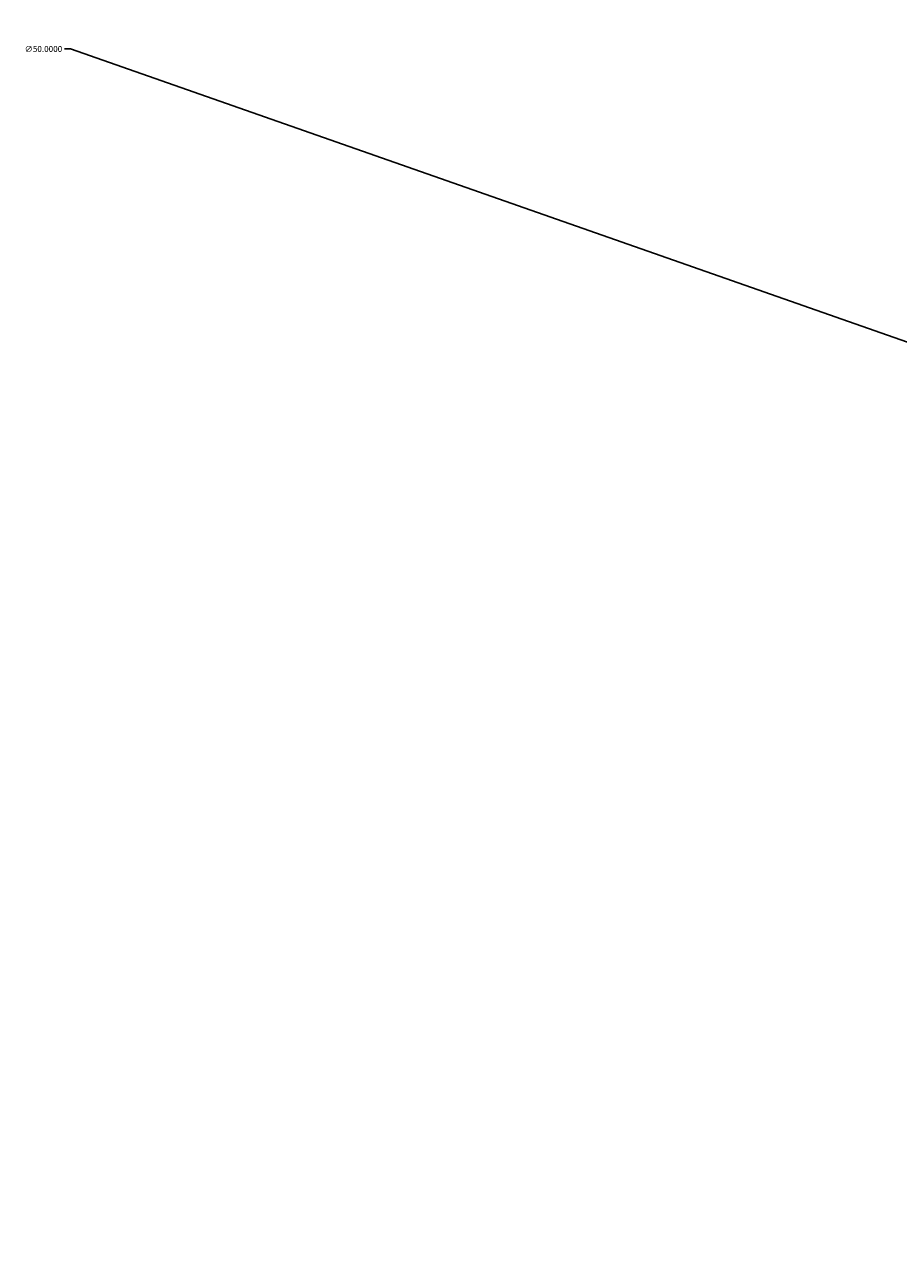
# Model space of a CAD drawing. Units: inches. Extents: x 139261 to 139415, y 52839 to 52963.
# Tile 3 of 20: x 139261 to 139288, y 52891 to 52928. Entities that reach past the tile are written whole.
import ezdxf

# ---------------------------------------------------------------- set-up
doc = ezdxf.new("R2010")
doc.units = ezdxf.units.IN
doc.header["$MEASUREMENT"] = 0
doc.layers.add('M-DIMS', color=2, linetype='Continuous', lineweight=25)
doc.styles.get("Standard").update_dxf_attribs({"font": 'arial.ttf'})
doc.dimstyles.get("Standard").update_dxf_attribs({"dimtxt": 0.18, "dimasz": 0.18, "dimexe": 0.18, "dimexo": 0.0625, "dimgap": 0.09, "dimtad": 0, "dimtih": 1, "dimtoh": 1, "dimdec": 4, "dimzin": 0, "dimdsep": 46, "dimtxsty": 'Standard', "dimcen": 0.09, "dimadec": 0, "dimazin": 0, "dimtfac": 1, "dimtdec": 4, "dimtofl": 0, "dimtmove": 0, "dimatfit": 3, "dimfxl": 1, "dimtolj": 1, "dimtzin": 0, "dimarcsym": 0})

# ---------------------------------------------------------------- blocks, each defined once
blk = doc.blocks.new('*D5')
at = {"layer": 'Defpoints', "color": 0, "transparency": 16777216}
for p in [(139316.763, 52908.484), (139363.951, 52891.951)]:
    blk.add_point(p, dxfattribs=at)
at = {"layer": 'M-DIMS', "color": 0, "lineweight": -2, "transparency": 16777216}
for p, q in [((139262.553, 52927.414), (139262.733, 52927.414)), ((139262.733, 52927.414), (139316.593, 52908.544)), ((139340.267, 52900.217), (139340.447, 52900.217)), ((139340.357, 52900.127), (139340.357, 52900.307))]:
    blk.add_line(p, q, dxfattribs=at)
at = {"layer": 'M-DIMS', "color": 0, "transparency": 16777216}
blk.add_solid([(139316.603, 52908.572), (139316.583, 52908.515), (139316.763, 52908.484)], dxfattribs=at)
at = {"layer": 'M-DIMS', "color": 0, "transparency": 16777216, "insert": (139261.922, 52927.414), "char_height": 0.18, "attachment_point": 5}
blk.add_mtext('\\A1;∅50.0000', dxfattribs=at)
blk = doc.blocks.new('*D9')
at = {"layer": 'Defpoints', "color": 0, "transparency": 16777216}
for p in [(139302.054, 52932.357), (139378.659, 52868.078)]:
    blk.add_point(p, dxfattribs=at)
at = {"layer": 'M-DIMS', "color": 0, "lineweight": -2, "transparency": 16777216}
for p, q in [((139278.893, 52951.64), (139279.073, 52951.64)), ((139279.073, 52951.64), (139301.916, 52932.472)), ((139340.267, 52900.217), (139340.447, 52900.217)), ((139340.357, 52900.127), (139340.357, 52900.307))]:
    blk.add_line(p, q, dxfattribs=at)
at = {"layer": 'M-DIMS', "color": 0, "transparency": 16777216}
blk.add_solid([(139301.936, 52932.495), (139301.897, 52932.449), (139302.054, 52932.357)], dxfattribs=at)
at = {"layer": 'M-DIMS', "color": 0, "transparency": 16777216, "insert": (139278.506, 52951.64), "char_height": 0.18, "attachment_point": 5}
blk.add_mtext('\\A1;∅100', dxfattribs=at)

msp = doc.modelspace()

# ---------------------------------------------------------------- dimensions: what is measured, and where the dimension line sits
at = {"layer": 'M-DIMS'}
for p1, p2, override, picture, middle in [((139378.65939, 52868.07845), (139302.05438, 52932.35652), {"dimdec": 0, "dimlfac": 1, "dimrnd": 0, "dimzin": 0, "dimdsep": 46, "dimlunit": 2}, '*D9', (139278.50641, 52951.63995)), ((139363.95063, 52891.95098), (139316.76314, 52908.48399), {"dimclrd": 0, "dimclre": 0, "dimclrt": 0}, '*D5', (139261.92224, 52927.41429))]:
    dim = msp.add_diameter_dim_2p(p1=p1, p2=p2, dimstyle='Standard', override=override, dxfattribs=at)
    dim.commit()
    dim.dimension.update_dxf_attribs({"geometry": picture, "text_midpoint": middle, "dimtype": 163})

doc.saveas('drawing.dxf')
